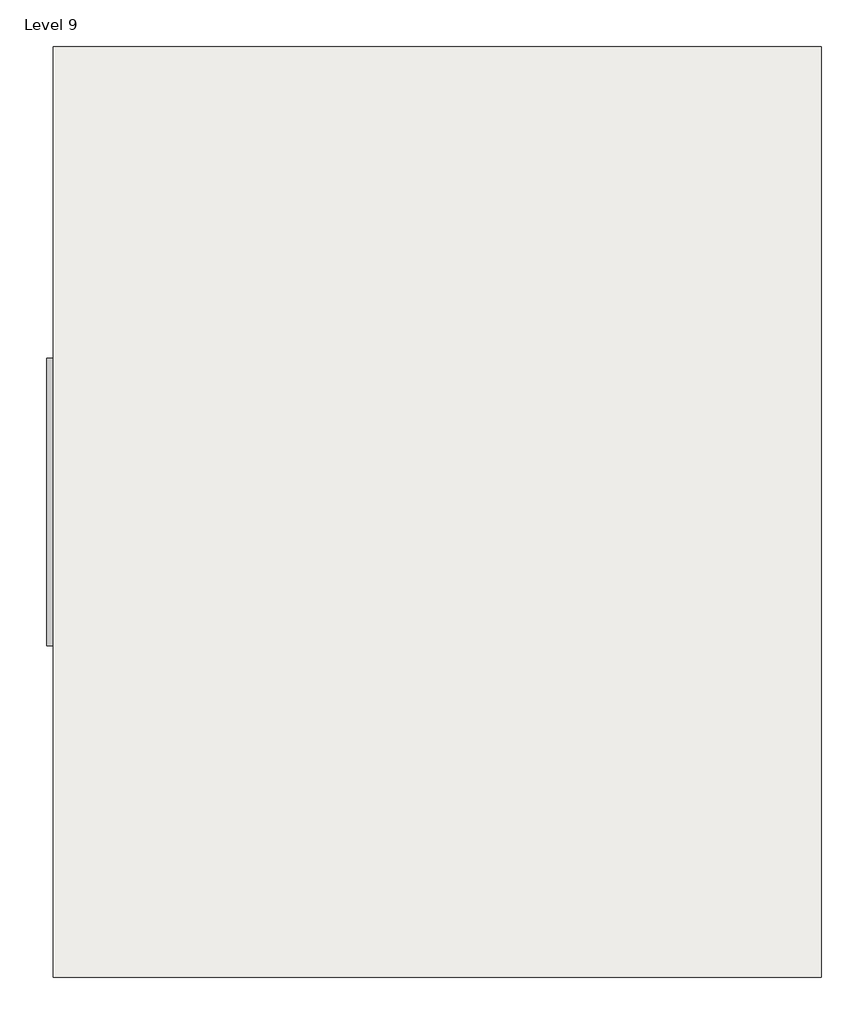
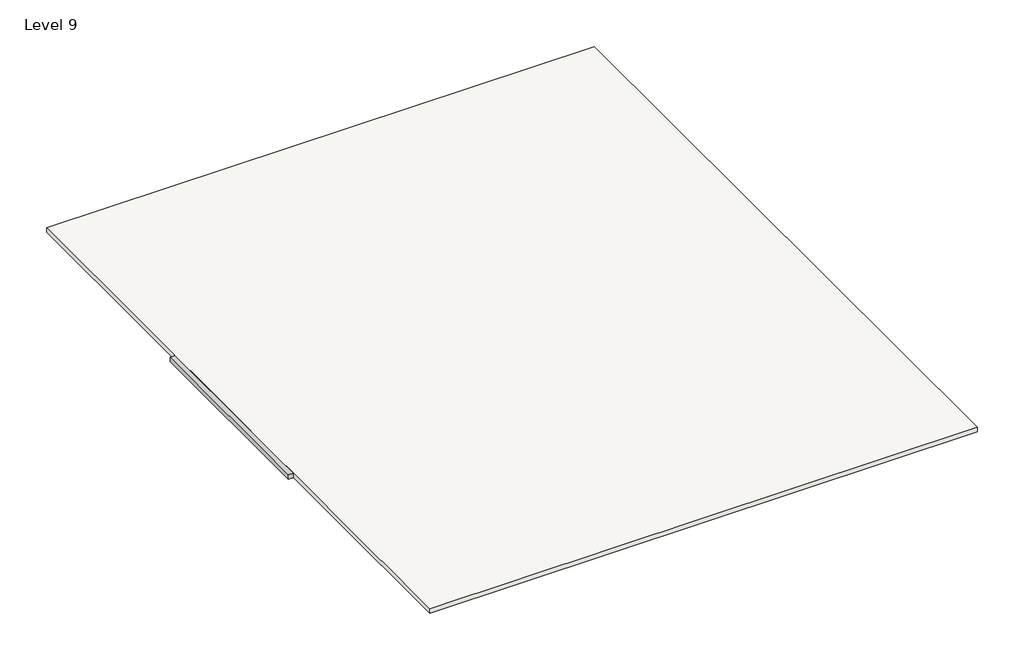
# One storey: 1 proxy, 1 slab.
"""IFC4 building model written with IfcOpenShell, lengths in millimetres."""

from ifc_helpers import new_model, si_unit, frame, origin, place, context, project, spatial, polyline, outline, extrude, transform, mapped, element, save
from components import generic_models_19_generic_models_19_fbad5572

model = new_model("IFC4")

# Units and contexts
model_context = context("Model", 3, world=origin())
ifc_project = project(units=[si_unit("LENGTHUNIT", "METRE", prefix="MILLI")], contexts=[model_context])

# Site, building, storey
site = spatial("IfcSite", under=ifc_project)
building = spatial("IfcBuilding", under=site)
storey = spatial("IfcBuildingStorey", under=building, Name="Level 9", Elevation=16154.4)

# Proxy
placement = place(None, origin())
generic_models_19_generic_models_19_shape = generic_models_19_generic_models_19_fbad5572(model_context)
element("IfcBuildingElementProxy", 1, Name="Generic Models 19 : Generic Models 19", ObjectType="Generic Models 19 : Generic Models 19", at=placement, inside=storey, context=model_context, shape_type="MappedRepresentation", body=[
    mapped(generic_models_19_generic_models_19_shape, transform((0.0, 0.0, 0.0), x_axis=(1.0, 0.0, 0.0), y_axis=(0.0, 1.0, 0.0), z_axis=(0.0, 0.0, 1.0))),
])

# Slab
element("IfcSlab", 2, ObjectType="Generic - 12\"", at=placement, inside=storey, context=model_context, shape_type="SweptSolid", body=[
    extrude(outline(polyline([(19165.761926, 20911.8014639), (19165.761926, -20845.7985361), (-15276.638074, -20845.7985361), (-15276.638074, 20911.8014639), (19165.761926, 20911.8014639)])), frame((0.0, 0.0, 16154.4), z_axis=(0.0, 0.0, 1.0), x_axis=(1.0, 0.0, 0.0)), (0.0, 0.0, 1.0), 304.8),
])

save(model, "model.ifc")

# Revit data of these elements
# Type "Generic - 12\""
#   Assembly Code = "B1010"
#   Function = 0
#   Layers, outside or top first: 1' - 0" no material (function 1)
# Element 1 (IfcBuildingElementProxy, "Generic Models 19 : Generic Models 19")
#   Phase Created = New Construction
# Element 2 (IfcSlab, "Generic - 12\"")
#   Height Offset From Level = 1' - 0"
#   Phase Created = New Construction
#   Materials on its faces: "Default Floor"
# Materials
#   "Default Floor": colour RGB 128 128 128, transparency 0
